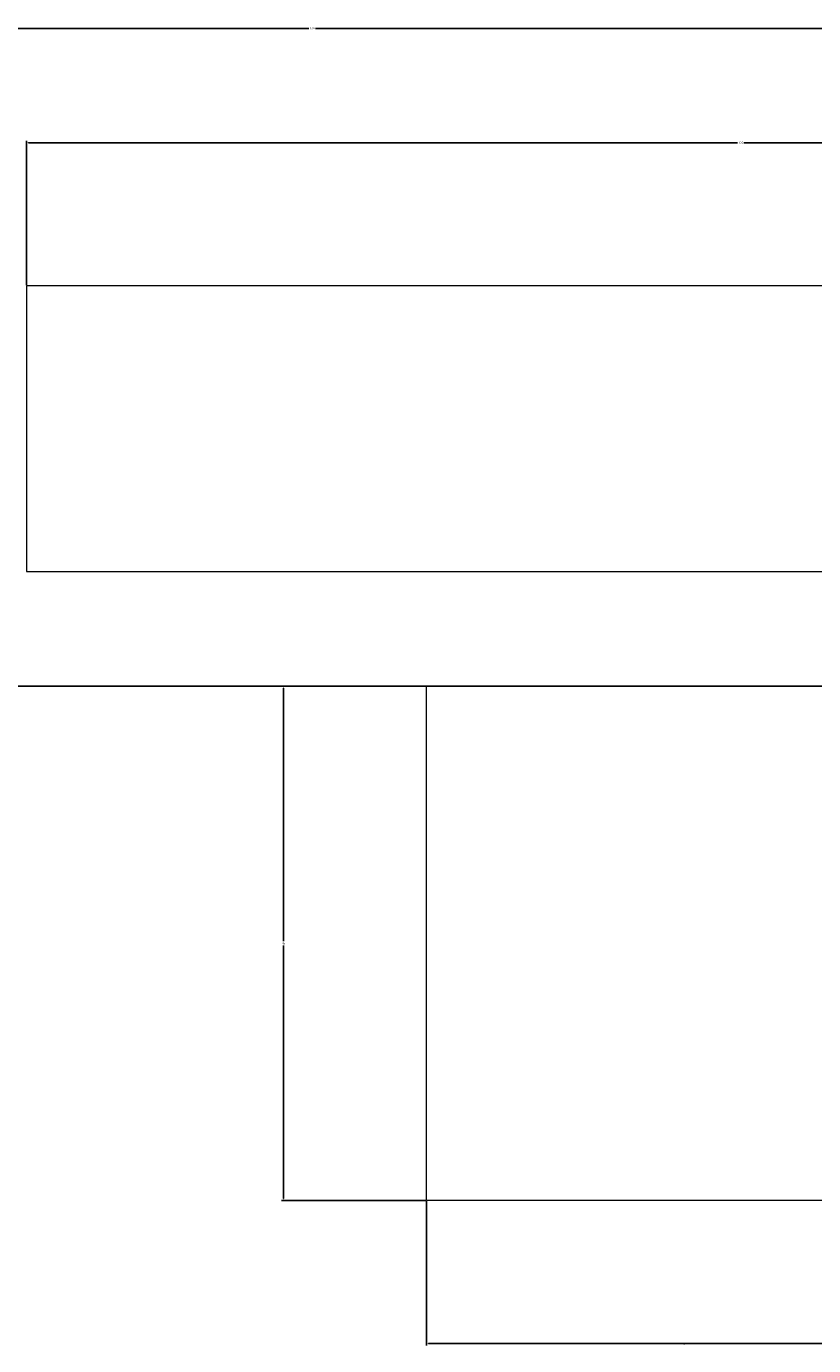
# Model space of a CAD drawing. Units: millimetres. Extents: x 135 to 361, y -58 to 58.
# Tile 3 of 5: x 223 to 292, y -58 to 58. Entities that reach past the tile are written whole.
import ezdxf

# ---------------------------------------------------------------- set-up
doc = ezdxf.new("R2010")
doc.units = ezdxf.units.MM
doc.layers.add('M-CONS', color=8, linetype='Continuous', lineweight=13)
doc.layers.add('M-DIMS', color=2, linetype='Continuous', lineweight=18)
doc.styles.get("Standard").update_dxf_attribs({"font": 'arial.ttf'})
doc.dimstyles.get("Standard").update_dxf_attribs({"dimtxt": 0.18, "dimasz": 0.18, "dimexe": 0.18, "dimexo": 0.0625, "dimgap": 0.09, "dimtad": 0, "dimtih": 1, "dimtoh": 1, "dimdec": 4, "dimzin": 0, "dimdsep": 46, "dimtxsty": 'Standard', "dimcen": 0.09, "dimadec": 0, "dimazin": 0, "dimtfac": 1, "dimtdec": 4, "dimtofl": 0, "dimtmove": 0, "dimatfit": 3, "dimfxl": 1, "dimtolj": 1, "dimtzin": 0, "dimarcsym": 0})

# ---------------------------------------------------------------- blocks, each defined once
blk = doc.blocks.new('*D1')
at = {"layer": 'Defpoints', "color": 0, "transparency": 16777216}
for p in [(347.81, 57.5), (347.81, 45), (147.81, 35)]:
    blk.add_point(p, dxfattribs=at)
at = {"layer": 'M-DIMS', "color": 0, "lineweight": -2, "transparency": 16777216}
for p, q in [((147.81, 35.06), (147.81, 57.68)), ((347.81, 45.06), (347.81, 57.68)), ((147.99, 57.5), (247.52, 57.5)), ((347.63, 57.5), (248.1, 57.5))]:
    blk.add_line(p, q, dxfattribs=at)
at = {"layer": 'M-DIMS', "color": 0, "transparency": 16777216}
for points in [[(147.99, 57.53), (147.99, 57.47), (147.81, 57.5)], [(347.63, 57.53), (347.63, 57.47), (347.81, 57.5)]]:
    blk.add_solid(points, dxfattribs=at)
at = {"layer": 'M-DIMS', "color": 0, "transparency": 16777216, "insert": (247.81, 57.5), "char_height": 0.18, "attachment_point": 5}
blk.add_mtext('\\A1;200', dxfattribs=at)
blk = doc.blocks.new('*D3')
at = {"layer": 'Defpoints', "color": 0, "transparency": 16777216}
for p in [(347.81, 47.5), (222.81, 35), (347.81, 35)]:
    blk.add_point(p, dxfattribs=at)
at = {"layer": 'M-DIMS', "color": 0, "lineweight": -2, "transparency": 16777216}
for p, q in [((222.81, 35.06), (222.81, 47.68)), ((222.99, 47.5), (285.03, 47.5)), ((347.63, 47.5), (285.59, 47.5)), ((347.81, 35.06), (347.81, 47.68))]:
    blk.add_line(p, q, dxfattribs=at)
at = {"layer": 'M-DIMS', "color": 0, "transparency": 16777216}
for points in [[(222.99, 47.53), (222.99, 47.47), (222.81, 47.5)], [(347.63, 47.53), (347.63, 47.47), (347.81, 47.5)]]:
    blk.add_solid(points, dxfattribs=at)
at = {"layer": 'M-DIMS', "color": 0, "transparency": 16777216, "insert": (285.31, 47.5), "char_height": 0.18, "attachment_point": 5}
blk.add_mtext('\\A1;125', dxfattribs=at)
blk = doc.blocks.new('*D6')
at = {"layer": 'Defpoints', "color": 0, "transparency": 16777216}
for p in [(257.81, -45), (347.81, -45), (347.81, -57.5)]:
    blk.add_point(p, dxfattribs=at)
at = {"layer": 'M-DIMS', "color": 0, "lineweight": -2, "transparency": 16777216}
for p, q in [((257.81, -45.06), (257.81, -57.68)), ((347.81, -45.06), (347.81, -57.68)), ((257.99, -57.5), (302.59, -57.5)), ((347.63, -57.5), (303.03, -57.5))]:
    blk.add_line(p, q, dxfattribs=at)
at = {"layer": 'M-DIMS', "color": 0, "transparency": 16777216}
for points in [[(257.99, -57.47), (257.99, -57.53), (257.81, -57.5)], [(347.63, -57.47), (347.63, -57.53), (347.81, -57.5)]]:
    blk.add_solid(points, dxfattribs=at)
at = {"layer": 'M-DIMS', "color": 0, "transparency": 16777216, "insert": (302.81, -57.5), "char_height": 0.18, "attachment_point": 5}
blk.add_mtext('\\A1;90', dxfattribs=at)
blk = doc.blocks.new('*D7')
at = {"layer": 'Defpoints', "color": 0, "transparency": 16777216}
for p in [(257.81, 0), (245.31, 0), (257.81, -45)]:
    blk.add_point(p, dxfattribs=at)
at = {"layer": 'M-DIMS', "color": 0, "lineweight": -2, "transparency": 16777216}
for p, q in [((257.75, 0), (245.13, 0)), ((245.31, -0.18), (245.31, -22.32)), ((245.31, -44.82), (245.31, -22.68)), ((257.75, -45), (245.13, -45))]:
    blk.add_line(p, q, dxfattribs=at)
at = {"layer": 'M-DIMS', "color": 0, "transparency": 16777216}
for points in [[(245.28, -0.18), (245.34, -0.18), (245.31, 0)], [(245.28, -44.82), (245.34, -44.82), (245.31, -45)]]:
    blk.add_solid(points, dxfattribs=at)
at = {"layer": 'M-DIMS', "color": 0, "transparency": 16777216, "insert": (245.31, -22.5), "char_height": 0.18, "attachment_point": 5}
blk.add_mtext('\\A1;45', dxfattribs=at)
blk = doc.blocks.new('*D8')
at = {"layer": 'Defpoints', "color": 0, "transparency": 16777216}
for p in [(302.81, -22.5), (257.81, -45), (302.81, -57.5)]:
    blk.add_point(p, dxfattribs=at)
at = {"layer": 'M-DIMS', "color": 0, "lineweight": -2, "transparency": 16777216}
for p, q in [((302.81, -22.56), (302.81, -57.68)), ((257.81, -45.06), (257.81, -57.68)), ((257.99, -57.5), (280.09, -57.5)), ((302.63, -57.5), (280.54, -57.5))]:
    blk.add_line(p, q, dxfattribs=at)
at = {"layer": 'M-DIMS', "color": 0, "transparency": 16777216}
for points in [[(257.99, -57.47), (257.99, -57.53), (257.81, -57.5)], [(302.63, -57.47), (302.63, -57.53), (302.81, -57.5)]]:
    blk.add_solid(points, dxfattribs=at)
at = {"layer": 'M-DIMS', "color": 0, "transparency": 16777216, "insert": (280.31, -57.5), "char_height": 0.18, "attachment_point": 5}
blk.add_mtext('\\A1;45', dxfattribs=at)

msp = doc.modelspace()

# ---------------------------------------------------------------- linework, layer by layer
at = {"layer": 'M-CONS', "elevation": 93.74}
for points in [[(347.81, 10), (347.81, 35), (222.81, 35), (222.81, 10)], [(347.81, -45), (257.81, -45), (257.81, 0), (347.81, 0)]]:
    msp.add_lwpolyline(points, close=True, dxfattribs=at)
at = {"layer": 'M-CONS', "extrusion": (0, -1, 0)}
msp.add_lwpolyline([(167.81, 133.74), (284.81, 145.74), (347.81, 117.74), (347.81, 93.74), (167.81, 93.74)], dxfattribs=at)

# ---------------------------------------------------------------- dimensions: what is measured, and where the dimension line sits
at = {"layer": 'M-DIMS'}
for base, p1, p2, picture, middle in [((347.81, 57.5), (147.81, 35), (347.81, 45), '*D1', (247.81, 57.5)), ((347.81, 47.5), (222.81, 35), (347.81, 35), '*D3', (285.31, 47.5)), ((302.81, -57.5), (257.81, -45), (302.81, -22.5), '*D8', (280.31, -57.5)), ((347.81, -57.5), (257.81, -45), (347.81, -45), '*D6', (302.81, -57.5))]:
    dim = msp.add_linear_dim(base=base, p1=p1, p2=p2, dimstyle='Standard', override={"dimdec": 0, "dimlfac": 1, "dimrnd": 0, "dimzin": 0, "dimdsep": 46, "dimlunit": 2}, dxfattribs=at)
    dim.commit()
    dim.dimension.update_dxf_attribs({"geometry": picture, "text_midpoint": middle})
dim = msp.add_linear_dim(base=(245.31, 0), p1=(257.81, -45), p2=(257.81, 0), angle=90, dimstyle='Standard', override={"dimdec": 0, "dimlfac": 1, "dimrnd": 0, "dimzin": 0, "dimdsep": 46, "dimlunit": 2}, dxfattribs=at)
dim.commit()
dim.dimension.update_dxf_attribs({"geometry": '*D7', "text_midpoint": (245.31, -22.5)})

doc.saveas('drawing.dxf')
